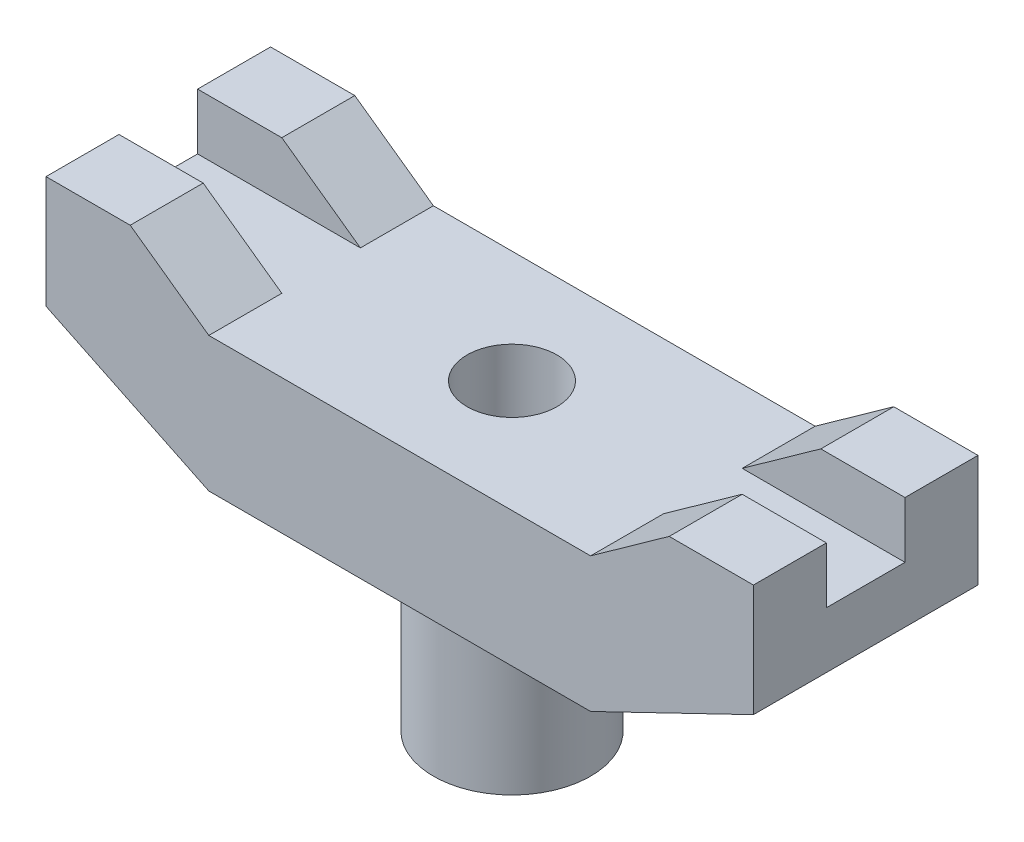
ISO-10303-21;
HEADER;
FILE_DESCRIPTION(('STEP AP214'),'2;1');
FILE_NAME('part.step','',(''),(''),'','','');
FILE_SCHEMA(('AUTOMOTIVE_DESIGN { 1 0 10303 214 1 1 1 1 }'));
ENDSEC;
DATA;
#1=APPLICATION_CONTEXT('core data for automotive mechanical design processes');
#2=APPLICATION_PROTOCOL_DEFINITION('international standard','automotive_design',2000,#1);
#3=PRODUCT_CONTEXT('',#1,'mechanical');
#4=PRODUCT('Part','Part','',(#3));
#5=PRODUCT_RELATED_PRODUCT_CATEGORY('part','',(#4));
#6=PRODUCT_DEFINITION_FORMATION('','',#4);
#7=PRODUCT_DEFINITION_CONTEXT('part definition',#1,'design');
#8=PRODUCT_DEFINITION('design','',#6,#7);
#9=PRODUCT_DEFINITION_SHAPE('','',#8);
#10=(LENGTH_UNIT() NAMED_UNIT(*) SI_UNIT(.MILLI.,.METRE.));
#11=(NAMED_UNIT(*) PLANE_ANGLE_UNIT() SI_UNIT($,.RADIAN.));
#12=(NAMED_UNIT(*) SI_UNIT($,.STERADIAN.) SOLID_ANGLE_UNIT());
#13=UNCERTAINTY_MEASURE_WITH_UNIT(LENGTH_MEASURE(1.E-05),#10,'distance_accuracy_value','');
#14=(GEOMETRIC_REPRESENTATION_CONTEXT(3) GLOBAL_UNCERTAINTY_ASSIGNED_CONTEXT((#13)) GLOBAL_UNIT_ASSIGNED_CONTEXT((#10,
#11,#12)) REPRESENTATION_CONTEXT('',''));
#15=CARTESIAN_POINT('',(0.,0.,0.));
#16=DIRECTION('',(0.,0.,1.));
#17=DIRECTION('',(1.,0.,0.));
#18=AXIS2_PLACEMENT_3D('',#15,#16,#17);
#19=CARTESIAN_POINT('',(0.,5.,0.));
#20=DIRECTION('',(0.,1.,0.));
#21=DIRECTION('',(0.,0.,1.));
#22=AXIS2_PLACEMENT_3D('',#19,#20,#21);
#23=PLANE('',#22);
#24=DIRECTION('',(-1.,0.,0.));
#25=VECTOR('',#24,1.);
#26=CARTESIAN_POINT('',(63.,5.,13.5));
#27=LINE('',#26,#25);
#28=CARTESIAN_POINT('',(7.5,5.,13.5));
#29=VERTEX_POINT('',#28);
#30=CARTESIAN_POINT('',(0.,5.,13.5));
#31=VERTEX_POINT('',#30);
#32=EDGE_CURVE('E211',#29,#31,#27,.T.);
#33=ORIENTED_EDGE('',*,*,#32,.T.);
#34=DIRECTION('',(0.,0.,1.));
#35=VECTOR('',#34,1.);
#36=CARTESIAN_POINT('',(0.,5.,0.));
#37=LINE('',#36,#35);
#38=CARTESIAN_POINT('',(0.,5.,20.));
#39=VERTEX_POINT('',#38);
#40=EDGE_CURVE('E257',#31,#39,#37,.T.);
#41=ORIENTED_EDGE('',*,*,#40,.T.);
#42=DIRECTION('',(-1.,0.,0.));
#43=VECTOR('',#42,1.);
#44=CARTESIAN_POINT('',(0.,5.,20.));
#45=LINE('',#44,#43);
#46=CARTESIAN_POINT('',(7.5,5.,20.));
#47=VERTEX_POINT('',#46);
#48=EDGE_CURVE('E248',#47,#39,#45,.T.);
#49=ORIENTED_EDGE('',*,*,#48,.F.);
#50=DIRECTION('',(0.,0.,1.));
#51=VECTOR('',#50,1.);
#52=CARTESIAN_POINT('',(7.5,5.,0.));
#53=LINE('',#52,#51);
#54=EDGE_CURVE('E262',#29,#47,#53,.T.);
#55=ORIENTED_EDGE('',*,*,#54,.F.);
#56=EDGE_LOOP('',(#33,#41,#49,#55));
#57=FACE_BOUND('',#56,.T.);
#58=ADVANCED_FACE('F44',(#57),#23,.T.);
#59=CARTESIAN_POINT('',(14.5,0.,0.));
#60=DIRECTION('',(0.581238193719096,0.813733471206735,0.));
#61=DIRECTION('',(-0.813733471206735,0.581238193719096,0.));
#62=AXIS2_PLACEMENT_3D('',#59,#60,#61);
#63=PLANE('',#62);
#64=DIRECTION('',(0.813733471206735,-0.581238193719096,0.));
#65=VECTOR('',#64,1.);
#66=CARTESIAN_POINT('',(14.5,0.,13.5));
#67=LINE('',#66,#65);
#68=CARTESIAN_POINT('',(14.5,0.,13.5));
#69=VERTEX_POINT('',#68);
#70=EDGE_CURVE('E219',#29,#69,#67,.T.);
#71=ORIENTED_EDGE('',*,*,#70,.F.);
#72=ORIENTED_EDGE('',*,*,#54,.T.);
#73=DIRECTION('',(-0.813733471206735,0.581238193719096,0.));
#74=VECTOR('',#73,1.);
#75=CARTESIAN_POINT('',(14.5,0.,20.));
#76=LINE('',#75,#74);
#77=CARTESIAN_POINT('',(14.5,0.,20.));
#78=VERTEX_POINT('',#77);
#79=EDGE_CURVE('E240',#78,#47,#76,.T.);
#80=ORIENTED_EDGE('',*,*,#79,.F.);
#81=DIRECTION('',(0.,0.,1.));
#82=VECTOR('',#81,1.);
#83=CARTESIAN_POINT('',(14.5,0.,0.));
#84=LINE('',#83,#82);
#85=EDGE_CURVE('E253',#69,#78,#84,.T.);
#86=ORIENTED_EDGE('',*,*,#85,.F.);
#87=EDGE_LOOP('',(#71,#72,#80,#86));
#88=FACE_BOUND('',#87,.T.);
#89=ADVANCED_FACE('F343',(#88),#63,.T.);
#90=CARTESIAN_POINT('',(48.5,0.,0.));
#91=DIRECTION('',(-0.581238193719096,0.813733471206735,0.));
#92=DIRECTION('',(-0.813733471206735,-0.581238193719096,0.));
#93=AXIS2_PLACEMENT_3D('',#90,#91,#92);
#94=PLANE('',#93);
#95=DIRECTION('',(0.813733471206735,0.581238193719096,0.));
#96=VECTOR('',#95,1.);
#97=CARTESIAN_POINT('',(48.5,0.,13.5));
#98=LINE('',#97,#96);
#99=CARTESIAN_POINT('',(48.5,0.,13.5));
#100=VERTEX_POINT('',#99);
#101=CARTESIAN_POINT('',(55.5,5.,13.5));
#102=VERTEX_POINT('',#101);
#103=EDGE_CURVE('E217',#100,#102,#98,.T.);
#104=ORIENTED_EDGE('',*,*,#103,.F.);
#105=DIRECTION('',(0.,0.,1.));
#106=VECTOR('',#105,1.);
#107=CARTESIAN_POINT('',(48.5,0.,0.));
#108=LINE('',#107,#106);
#109=CARTESIAN_POINT('',(48.5,0.,20.));
#110=VERTEX_POINT('',#109);
#111=EDGE_CURVE('E236',#100,#110,#108,.T.);
#112=ORIENTED_EDGE('',*,*,#111,.T.);
#113=DIRECTION('',(-0.813733471206735,-0.581238193719096,0.));
#114=VECTOR('',#113,1.);
#115=CARTESIAN_POINT('',(48.5,0.,20.));
#116=LINE('',#115,#114);
#117=CARTESIAN_POINT('',(55.5,5.,20.));
#118=VERTEX_POINT('',#117);
#119=EDGE_CURVE('E230',#118,#110,#116,.T.);
#120=ORIENTED_EDGE('',*,*,#119,.F.);
#121=DIRECTION('',(0.,0.,1.));
#122=VECTOR('',#121,1.);
#123=CARTESIAN_POINT('',(55.5,5.,0.));
#124=LINE('',#123,#122);
#125=EDGE_CURVE('E245',#102,#118,#124,.T.);
#126=ORIENTED_EDGE('',*,*,#125,.F.);
#127=EDGE_LOOP('',(#104,#112,#120,#126));
#128=FACE_BOUND('',#127,.T.);
#129=ADVANCED_FACE('F348',(#128),#94,.T.);
#130=CARTESIAN_POINT('',(63.,5.,0.));
#131=DIRECTION('',(0.,1.,0.));
#132=DIRECTION('',(0.,0.,1.));
#133=AXIS2_PLACEMENT_3D('',#130,#131,#132);
#134=PLANE('',#133);
#135=CARTESIAN_POINT('',(63.,5.,13.5));
#136=VERTEX_POINT('',#135);
#137=EDGE_CURVE('E208',#136,#102,#27,.T.);
#138=ORIENTED_EDGE('',*,*,#137,.T.);
#139=ORIENTED_EDGE('',*,*,#125,.T.);
#140=DIRECTION('',(-1.,0.,0.));
#141=VECTOR('',#140,1.);
#142=CARTESIAN_POINT('',(63.,5.,20.));
#143=LINE('',#142,#141);
#144=CARTESIAN_POINT('',(63.,5.,20.));
#145=VERTEX_POINT('',#144);
#146=EDGE_CURVE('E225',#145,#118,#143,.T.);
#147=ORIENTED_EDGE('',*,*,#146,.F.);
#148=DIRECTION('',(0.,0.,1.));
#149=VECTOR('',#148,1.);
#150=CARTESIAN_POINT('',(63.,5.,0.));
#151=LINE('',#150,#149);
#152=EDGE_CURVE('E229',#136,#145,#151,.T.);
#153=ORIENTED_EDGE('',*,*,#152,.F.);
#154=EDGE_LOOP('',(#138,#139,#147,#153));
#155=FACE_BOUND('',#154,.T.);
#156=ADVANCED_FACE('F354',(#155),#134,.T.);
#157=CARTESIAN_POINT('',(0.,0.,20.));
#158=DIRECTION('',(1.,0.,0.));
#159=DIRECTION('',(0.,0.,-1.));
#160=AXIS2_PLACEMENT_3D('',#157,#158,#159);
#161=PLANE('',#160);
#162=ORIENTED_EDGE('',*,*,#40,.F.);
#163=DIRECTION('',(0.,1.,0.));
#164=VECTOR('',#163,1.);
#165=CARTESIAN_POINT('',(0.,0.,13.5));
#166=LINE('',#165,#164);
#167=CARTESIAN_POINT('',(0.,0.,13.5));
#168=VERTEX_POINT('',#167);
#169=EDGE_CURVE('E191',#168,#31,#166,.T.);
#170=ORIENTED_EDGE('',*,*,#169,.F.);
#171=DIRECTION('',(0.,0.,1.));
#172=VECTOR('',#171,1.);
#173=CARTESIAN_POINT('',(0.,0.,6.5));
#174=LINE('',#173,#172);
#175=CARTESIAN_POINT('',(0.,0.,6.5));
#176=VERTEX_POINT('',#175);
#177=EDGE_CURVE('E197',#176,#168,#174,.T.);
#178=ORIENTED_EDGE('',*,*,#177,.F.);
#179=DIRECTION('',(0.,-1.,0.));
#180=VECTOR('',#179,1.);
#181=CARTESIAN_POINT('',(0.,5.,6.5));
#182=LINE('',#181,#180);
#183=CARTESIAN_POINT('',(0.,5.,6.5));
#184=VERTEX_POINT('',#183);
#185=EDGE_CURVE('E201',#184,#176,#182,.T.);
#186=ORIENTED_EDGE('',*,*,#185,.F.);
#187=CARTESIAN_POINT('',(0.,5.,0.));
#188=VERTEX_POINT('',#187);
#189=EDGE_CURVE('E258',#188,#184,#37,.T.);
#190=ORIENTED_EDGE('',*,*,#189,.F.);
#191=DIRECTION('',(0.,-1.,0.));
#192=VECTOR('',#191,1.);
#193=CARTESIAN_POINT('',(0.,0.,0.));
#194=LINE('',#193,#192);
#195=CARTESIAN_POINT('',(0.,-5.,0.));
#196=VERTEX_POINT('',#195);
#197=EDGE_CURVE('E259',#188,#196,#194,.T.);
#198=ORIENTED_EDGE('',*,*,#197,.T.);
#199=DIRECTION('',(0.,0.,-1.));
#200=VECTOR('',#199,1.);
#201=CARTESIAN_POINT('',(0.,-5.,20.));
#202=LINE('',#201,#200);
#203=CARTESIAN_POINT('',(0.,-5.,20.));
#204=VERTEX_POINT('',#203);
#205=EDGE_CURVE('E53',#204,#196,#202,.T.);
#206=ORIENTED_EDGE('',*,*,#205,.F.);
#207=DIRECTION('',(0.,-1.,0.));
#208=VECTOR('',#207,1.);
#209=CARTESIAN_POINT('',(0.,0.,20.));
#210=LINE('',#209,#208);
#211=EDGE_CURVE('E270',#39,#204,#210,.T.);
#212=ORIENTED_EDGE('',*,*,#211,.F.);
#213=EDGE_LOOP('',(#162,#170,#178,#186,#190,#198,#206,#212));
#214=FACE_BOUND('',#213,.T.);
#215=ADVANCED_FACE('F50',(#214),#161,.F.);
#216=CARTESIAN_POINT('',(0.,-5.,20.));
#217=DIRECTION('',(0.434749065831176,0.900551636364578,0.));
#218=DIRECTION('',(-0.900551636364579,0.434749065831176,0.));
#219=AXIS2_PLACEMENT_3D('',#216,#217,#218);
#220=PLANE('',#219);
#221=DIRECTION('',(0.900551636364578,-0.434749065831176,0.));
#222=VECTOR('',#221,1.);
#223=CARTESIAN_POINT('',(0.,-5.,0.));
#224=LINE('',#223,#222);
#225=CARTESIAN_POINT('',(14.5,-12.,0.));
#226=VERTEX_POINT('',#225);
#227=EDGE_CURVE('E287',#196,#226,#224,.T.);
#228=ORIENTED_EDGE('',*,*,#227,.T.);
#229=DIRECTION('',(0.,0.,-1.));
#230=VECTOR('',#229,1.);
#231=CARTESIAN_POINT('',(14.5,-12.,20.));
#232=LINE('',#231,#230);
#233=CARTESIAN_POINT('',(14.5,-12.,20.));
#234=VERTEX_POINT('',#233);
#235=EDGE_CURVE('E302',#234,#226,#232,.T.);
#236=ORIENTED_EDGE('',*,*,#235,.F.);
#237=DIRECTION('',(0.900551636364578,-0.434749065831176,0.));
#238=VECTOR('',#237,1.);
#239=CARTESIAN_POINT('',(0.,-5.,20.));
#240=LINE('',#239,#238);
#241=EDGE_CURVE('E269',#204,#234,#240,.T.);
#242=ORIENTED_EDGE('',*,*,#241,.F.);
#243=ORIENTED_EDGE('',*,*,#205,.T.);
#244=EDGE_LOOP('',(#228,#236,#242,#243));
#245=FACE_BOUND('',#244,.T.);
#246=ADVANCED_FACE('F308',(#245),#220,.F.);
#247=CARTESIAN_POINT('',(31.5,-12.,20.));
#248=DIRECTION('',(0.,1.,0.));
#249=DIRECTION('',(0.,0.,1.));
#250=AXIS2_PLACEMENT_3D('',#247,#248,#249);
#251=PLANE('',#250);
#252=CARTESIAN_POINT('',(31.5,-12.,10.));
#253=DIRECTION('',(0.,-1.,0.));
#254=DIRECTION('',(0.,0.,-1.));
#255=AXIS2_PLACEMENT_3D('',#252,#253,#254);
#256=CIRCLE('',#255,7.);
#257=CARTESIAN_POINT('',(31.5,-12.,3.));
#258=VERTEX_POINT('',#257);
#259=EDGE_CURVE('E11',#258,#258,#256,.T.);
#260=ORIENTED_EDGE('',*,*,#259,.F.);
#261=EDGE_LOOP('',(#260));
#262=FACE_BOUND('',#261,.T.);
#263=DIRECTION('',(1.,0.,0.));
#264=VECTOR('',#263,1.);
#265=CARTESIAN_POINT('',(31.5,-12.,0.));
#266=LINE('',#265,#264);
#267=CARTESIAN_POINT('',(48.5,-12.,0.));
#268=VERTEX_POINT('',#267);
#269=EDGE_CURVE('E289',#226,#268,#266,.T.);
#270=ORIENTED_EDGE('',*,*,#269,.T.);
#271=DIRECTION('',(0.,0.,-1.));
#272=VECTOR('',#271,1.);
#273=CARTESIAN_POINT('',(48.5,-12.,20.));
#274=LINE('',#273,#272);
#275=CARTESIAN_POINT('',(48.5,-12.,20.));
#276=VERTEX_POINT('',#275);
#277=EDGE_CURVE('E296',#276,#268,#274,.T.);
#278=ORIENTED_EDGE('',*,*,#277,.F.);
#279=DIRECTION('',(1.,0.,0.));
#280=VECTOR('',#279,1.);
#281=CARTESIAN_POINT('',(31.5,-12.,20.));
#282=LINE('',#281,#280);
#283=EDGE_CURVE('E272',#234,#276,#282,.T.);
#284=ORIENTED_EDGE('',*,*,#283,.F.);
#285=ORIENTED_EDGE('',*,*,#235,.T.);
#286=EDGE_LOOP('',(#270,#278,#284,#285));
#287=FACE_BOUND('',#286,.T.);
#288=ADVANCED_FACE('F321',(#262,#287),#251,.F.);
#289=CARTESIAN_POINT('',(63.,-5.,20.));
#290=DIRECTION('',(-0.434749065831176,0.900551636364578,0.));
#291=DIRECTION('',(-0.900551636364579,-0.434749065831176,0.));
#292=AXIS2_PLACEMENT_3D('',#289,#290,#291);
#293=PLANE('',#292);
#294=DIRECTION('',(0.900551636364578,0.434749065831176,0.));
#295=VECTOR('',#294,1.);
#296=CARTESIAN_POINT('',(63.,-5.,0.));
#297=LINE('',#296,#295);
#298=CARTESIAN_POINT('',(63.,-5.,0.));
#299=VERTEX_POINT('',#298);
#300=EDGE_CURVE('E292',#268,#299,#297,.T.);
#301=ORIENTED_EDGE('',*,*,#300,.T.);
#302=DIRECTION('',(0.,0.,-1.));
#303=VECTOR('',#302,1.);
#304=CARTESIAN_POINT('',(63.,-5.,20.));
#305=LINE('',#304,#303);
#306=CARTESIAN_POINT('',(63.,-5.,20.));
#307=VERTEX_POINT('',#306);
#308=EDGE_CURVE('E281',#307,#299,#305,.T.);
#309=ORIENTED_EDGE('',*,*,#308,.F.);
#310=DIRECTION('',(0.900551636364578,0.434749065831176,0.));
#311=VECTOR('',#310,1.);
#312=CARTESIAN_POINT('',(63.,-5.,20.));
#313=LINE('',#312,#311);
#314=EDGE_CURVE('E274',#276,#307,#313,.T.);
#315=ORIENTED_EDGE('',*,*,#314,.F.);
#316=ORIENTED_EDGE('',*,*,#277,.T.);
#317=EDGE_LOOP('',(#301,#309,#315,#316));
#318=FACE_BOUND('',#317,.T.);
#319=ADVANCED_FACE('F324',(#318),#293,.F.);
#320=CARTESIAN_POINT('',(63.,0.,20.));
#321=DIRECTION('',(-1.,0.,0.));
#322=DIRECTION('',(0.,0.,1.));
#323=AXIS2_PLACEMENT_3D('',#320,#321,#322);
#324=PLANE('',#323);
#325=DIRECTION('',(0.,0.,1.));
#326=VECTOR('',#325,1.);
#327=CARTESIAN_POINT('',(63.,0.,6.5));
#328=LINE('',#327,#326);
#329=CARTESIAN_POINT('',(63.,0.,6.5));
#330=VERTEX_POINT('',#329);
#331=CARTESIAN_POINT('',(63.,0.,13.5));
#332=VERTEX_POINT('',#331);
#333=EDGE_CURVE('E182',#330,#332,#328,.T.);
#334=ORIENTED_EDGE('',*,*,#333,.T.);
#335=DIRECTION('',(0.,1.,0.));
#336=VECTOR('',#335,1.);
#337=CARTESIAN_POINT('',(63.,0.,13.5));
#338=LINE('',#337,#336);
#339=EDGE_CURVE('E187',#332,#136,#338,.T.);
#340=ORIENTED_EDGE('',*,*,#339,.T.);
#341=ORIENTED_EDGE('',*,*,#152,.T.);
#342=DIRECTION('',(0.,1.,0.));
#343=VECTOR('',#342,1.);
#344=CARTESIAN_POINT('',(63.,0.,20.));
#345=LINE('',#344,#343);
#346=EDGE_CURVE('E280',#307,#145,#345,.T.);
#347=ORIENTED_EDGE('',*,*,#346,.F.);
#348=ORIENTED_EDGE('',*,*,#308,.T.);
#349=DIRECTION('',(0.,1.,0.));
#350=VECTOR('',#349,1.);
#351=CARTESIAN_POINT('',(63.,0.,0.));
#352=LINE('',#351,#350);
#353=CARTESIAN_POINT('',(63.,5.,0.));
#354=VERTEX_POINT('',#353);
#355=EDGE_CURVE('E291',#299,#354,#352,.T.);
#356=ORIENTED_EDGE('',*,*,#355,.T.);
#357=CARTESIAN_POINT('',(63.,5.,6.5));
#358=VERTEX_POINT('',#357);
#359=EDGE_CURVE('E194',#354,#358,#151,.T.);
#360=ORIENTED_EDGE('',*,*,#359,.T.);
#361=DIRECTION('',(0.,-1.,0.));
#362=VECTOR('',#361,1.);
#363=CARTESIAN_POINT('',(63.,5.,6.5));
#364=LINE('',#363,#362);
#365=EDGE_CURVE('E66',#358,#330,#364,.T.);
#366=ORIENTED_EDGE('',*,*,#365,.T.);
#367=EDGE_LOOP('',(#334,#340,#341,#347,#348,#356,#360,#366));
#368=FACE_BOUND('',#367,.T.);
#369=ADVANCED_FACE('F195',(#368),#324,.F.);
#370=CARTESIAN_POINT('',(0.,0.,20.));
#371=DIRECTION('',(0.,-1.,0.));
#372=DIRECTION('',(0.,0.,-1.));
#373=AXIS2_PLACEMENT_3D('',#370,#371,#372);
#374=PLANE('',#373);
#375=CARTESIAN_POINT('',(31.5,0.,10.));
#376=DIRECTION('',(0.,1.,0.));
#377=DIRECTION('',(0.,0.,1.));
#378=AXIS2_PLACEMENT_3D('',#375,#376,#377);
#379=CIRCLE('',#378,4.);
#380=CARTESIAN_POINT('',(31.5,0.,14.));
#381=VERTEX_POINT('',#380);
#382=EDGE_CURVE('E440',#381,#381,#379,.T.);
#383=ORIENTED_EDGE('',*,*,#382,.F.);
#384=EDGE_LOOP('',(#383));
#385=FACE_BOUND('',#384,.T.);
#386=CARTESIAN_POINT('',(14.5,0.,0.));
#387=VERTEX_POINT('',#386);
#388=CARTESIAN_POINT('',(14.5,0.,6.5));
#389=VERTEX_POINT('',#388);
#390=EDGE_CURVE('E264',#387,#389,#84,.T.);
#391=ORIENTED_EDGE('',*,*,#390,.T.);
#392=DIRECTION('',(-1.,0.,0.));
#393=VECTOR('',#392,1.);
#394=CARTESIAN_POINT('',(63.,0.,6.5));
#395=LINE('',#394,#393);
#396=EDGE_CURVE('E65',#389,#176,#395,.T.);
#397=ORIENTED_EDGE('',*,*,#396,.T.);
#398=ORIENTED_EDGE('',*,*,#177,.T.);
#399=DIRECTION('',(-1.,0.,0.));
#400=VECTOR('',#399,1.);
#401=CARTESIAN_POINT('',(63.,0.,13.5));
#402=LINE('',#401,#400);
#403=EDGE_CURVE('E178',#69,#168,#402,.T.);
#404=ORIENTED_EDGE('',*,*,#403,.F.);
#405=ORIENTED_EDGE('',*,*,#85,.T.);
#406=DIRECTION('',(-1.,0.,0.));
#407=VECTOR('',#406,1.);
#408=CARTESIAN_POINT('',(0.,0.,20.));
#409=LINE('',#408,#407);
#410=EDGE_CURVE('E278',#110,#78,#409,.T.);
#411=ORIENTED_EDGE('',*,*,#410,.F.);
#412=ORIENTED_EDGE('',*,*,#111,.F.);
#413=EDGE_CURVE('E183',#332,#100,#402,.T.);
#414=ORIENTED_EDGE('',*,*,#413,.F.);
#415=ORIENTED_EDGE('',*,*,#333,.F.);
#416=CARTESIAN_POINT('',(48.5,0.,6.5));
#417=VERTEX_POINT('',#416);
#418=EDGE_CURVE('E168',#330,#417,#395,.T.);
#419=ORIENTED_EDGE('',*,*,#418,.T.);
#420=CARTESIAN_POINT('',(48.5,0.,0.));
#421=VERTEX_POINT('',#420);
#422=EDGE_CURVE('E231',#421,#417,#108,.T.);
#423=ORIENTED_EDGE('',*,*,#422,.F.);
#424=DIRECTION('',(-1.,0.,0.));
#425=VECTOR('',#424,1.);
#426=CARTESIAN_POINT('',(0.,0.,0.));
#427=LINE('',#426,#425);
#428=EDGE_CURVE('E271',#421,#387,#427,.T.);
#429=ORIENTED_EDGE('',*,*,#428,.T.);
#430=EDGE_LOOP('',(#391,#397,#398,#404,#405,#411,#412,#414,#415,#419,#423,#429));
#431=FACE_BOUND('',#430,.T.);
#432=ADVANCED_FACE('F181',(#385,#431),#374,.F.);
#433=CARTESIAN_POINT('',(0.,0.,20.));
#434=DIRECTION('',(0.,0.,-1.));
#435=DIRECTION('',(-1.,0.,0.));
#436=AXIS2_PLACEMENT_3D('',#433,#434,#435);
#437=PLANE('',#436);
#438=ORIENTED_EDGE('',*,*,#211,.T.);
#439=ORIENTED_EDGE('',*,*,#241,.T.);
#440=ORIENTED_EDGE('',*,*,#283,.T.);
#441=ORIENTED_EDGE('',*,*,#314,.T.);
#442=ORIENTED_EDGE('',*,*,#346,.T.);
#443=ORIENTED_EDGE('',*,*,#146,.T.);
#444=ORIENTED_EDGE('',*,*,#119,.T.);
#445=ORIENTED_EDGE('',*,*,#410,.T.);
#446=ORIENTED_EDGE('',*,*,#79,.T.);
#447=ORIENTED_EDGE('',*,*,#48,.T.);
#448=EDGE_LOOP('',(#438,#439,#440,#441,#442,#443,#444,#445,#446,#447));
#449=FACE_BOUND('',#448,.T.);
#450=ADVANCED_FACE('F328',(#449),#437,.F.);
#451=CARTESIAN_POINT('',(0.,0.,0.));
#452=DIRECTION('',(0.,0.,-1.));
#453=DIRECTION('',(-1.,0.,0.));
#454=AXIS2_PLACEMENT_3D('',#451,#452,#453);
#455=PLANE('',#454);
#456=ORIENTED_EDGE('',*,*,#197,.F.);
#457=DIRECTION('',(-1.,0.,0.));
#458=VECTOR('',#457,1.);
#459=CARTESIAN_POINT('',(0.,5.,0.));
#460=LINE('',#459,#458);
#461=CARTESIAN_POINT('',(7.5,5.,0.));
#462=VERTEX_POINT('',#461);
#463=EDGE_CURVE('E250',#462,#188,#460,.T.);
#464=ORIENTED_EDGE('',*,*,#463,.F.);
#465=DIRECTION('',(-0.813733471206735,0.581238193719096,0.));
#466=VECTOR('',#465,1.);
#467=CARTESIAN_POINT('',(14.5,0.,0.));
#468=LINE('',#467,#466);
#469=EDGE_CURVE('E242',#387,#462,#468,.T.);
#470=ORIENTED_EDGE('',*,*,#469,.F.);
#471=ORIENTED_EDGE('',*,*,#428,.F.);
#472=DIRECTION('',(-0.813733471206735,-0.581238193719096,0.));
#473=VECTOR('',#472,1.);
#474=CARTESIAN_POINT('',(48.5,0.,0.));
#475=LINE('',#474,#473);
#476=CARTESIAN_POINT('',(55.5,5.,0.));
#477=VERTEX_POINT('',#476);
#478=EDGE_CURVE('E228',#477,#421,#475,.T.);
#479=ORIENTED_EDGE('',*,*,#478,.F.);
#480=DIRECTION('',(-1.,0.,0.));
#481=VECTOR('',#480,1.);
#482=CARTESIAN_POINT('',(63.,5.,0.));
#483=LINE('',#482,#481);
#484=EDGE_CURVE('E224',#354,#477,#483,.T.);
#485=ORIENTED_EDGE('',*,*,#484,.F.);
#486=ORIENTED_EDGE('',*,*,#355,.F.);
#487=ORIENTED_EDGE('',*,*,#300,.F.);
#488=ORIENTED_EDGE('',*,*,#269,.F.);
#489=ORIENTED_EDGE('',*,*,#227,.F.);
#490=EDGE_LOOP('',(#456,#464,#470,#471,#479,#485,#486,#487,#488,#489));
#491=FACE_BOUND('',#490,.T.);
#492=ADVANCED_FACE('F312',(#491),#455,.T.);
#493=DIRECTION('',(-1.,0.,0.));
#494=VECTOR('',#493,1.);
#495=CARTESIAN_POINT('',(63.,5.,6.5));
#496=LINE('',#495,#494);
#497=CARTESIAN_POINT('',(7.5,5.,6.5));
#498=VERTEX_POINT('',#497);
#499=EDGE_CURVE('E205',#498,#184,#496,.T.);
#500=ORIENTED_EDGE('',*,*,#499,.F.);
#501=EDGE_CURVE('E261',#462,#498,#53,.T.);
#502=ORIENTED_EDGE('',*,*,#501,.F.);
#503=ORIENTED_EDGE('',*,*,#463,.T.);
#504=ORIENTED_EDGE('',*,*,#189,.T.);
#505=EDGE_LOOP('',(#500,#502,#503,#504));
#506=FACE_BOUND('',#505,.T.);
#507=ADVANCED_FACE('F366',(#506),#23,.T.);
#508=DIRECTION('',(-0.813733471206735,0.581238193719096,0.));
#509=VECTOR('',#508,1.);
#510=CARTESIAN_POINT('',(14.5,0.,6.5));
#511=LINE('',#510,#509);
#512=EDGE_CURVE('E216',#389,#498,#511,.T.);
#513=ORIENTED_EDGE('',*,*,#512,.F.);
#514=ORIENTED_EDGE('',*,*,#390,.F.);
#515=ORIENTED_EDGE('',*,*,#469,.T.);
#516=ORIENTED_EDGE('',*,*,#501,.T.);
#517=EDGE_LOOP('',(#513,#514,#515,#516));
#518=FACE_BOUND('',#517,.T.);
#519=ADVANCED_FACE('F365',(#518),#63,.T.);
#520=DIRECTION('',(-0.813733471206735,-0.581238193719096,0.));
#521=VECTOR('',#520,1.);
#522=CARTESIAN_POINT('',(48.5,0.,6.5));
#523=LINE('',#522,#521);
#524=CARTESIAN_POINT('',(55.5,5.,6.5));
#525=VERTEX_POINT('',#524);
#526=EDGE_CURVE('E172',#525,#417,#523,.T.);
#527=ORIENTED_EDGE('',*,*,#526,.F.);
#528=EDGE_CURVE('E239',#477,#525,#124,.T.);
#529=ORIENTED_EDGE('',*,*,#528,.F.);
#530=ORIENTED_EDGE('',*,*,#478,.T.);
#531=ORIENTED_EDGE('',*,*,#422,.T.);
#532=EDGE_LOOP('',(#527,#529,#530,#531));
#533=FACE_BOUND('',#532,.T.);
#534=ADVANCED_FACE('F363',(#533),#94,.T.);
#535=EDGE_CURVE('E213',#358,#525,#496,.T.);
#536=ORIENTED_EDGE('',*,*,#535,.F.);
#537=ORIENTED_EDGE('',*,*,#359,.F.);
#538=ORIENTED_EDGE('',*,*,#484,.T.);
#539=ORIENTED_EDGE('',*,*,#528,.T.);
#540=EDGE_LOOP('',(#536,#537,#538,#539));
#541=FACE_BOUND('',#540,.T.);
#542=ADVANCED_FACE('F359',(#541),#134,.T.);
#543=CARTESIAN_POINT('',(63.,0.,13.5));
#544=DIRECTION('',(0.,0.,1.));
#545=DIRECTION('',(1.,0.,0.));
#546=AXIS2_PLACEMENT_3D('',#543,#544,#545);
#547=PLANE('',#546);
#548=ORIENTED_EDGE('',*,*,#103,.T.);
#549=ORIENTED_EDGE('',*,*,#137,.F.);
#550=ORIENTED_EDGE('',*,*,#339,.F.);
#551=ORIENTED_EDGE('',*,*,#413,.T.);
#552=EDGE_LOOP('',(#548,#549,#550,#551));
#553=FACE_BOUND('',#552,.T.);
#554=ADVANCED_FACE('F355',(#553),#547,.F.);
#555=CARTESIAN_POINT('',(63.,5.,6.5));
#556=DIRECTION('',(0.,0.,-1.));
#557=DIRECTION('',(-1.,0.,0.));
#558=AXIS2_PLACEMENT_3D('',#555,#556,#557);
#559=PLANE('',#558);
#560=ORIENTED_EDGE('',*,*,#526,.T.);
#561=ORIENTED_EDGE('',*,*,#418,.F.);
#562=ORIENTED_EDGE('',*,*,#365,.F.);
#563=ORIENTED_EDGE('',*,*,#535,.T.);
#564=EDGE_LOOP('',(#560,#561,#562,#563));
#565=FACE_BOUND('',#564,.T.);
#566=ADVANCED_FACE('F175',(#565),#559,.F.);
#567=ORIENTED_EDGE('',*,*,#70,.T.);
#568=ORIENTED_EDGE('',*,*,#403,.T.);
#569=ORIENTED_EDGE('',*,*,#169,.T.);
#570=ORIENTED_EDGE('',*,*,#32,.F.);
#571=EDGE_LOOP('',(#567,#568,#569,#570));
#572=FACE_BOUND('',#571,.T.);
#573=ADVANCED_FACE('F337',(#572),#547,.F.);
#574=ORIENTED_EDGE('',*,*,#512,.T.);
#575=ORIENTED_EDGE('',*,*,#499,.T.);
#576=ORIENTED_EDGE('',*,*,#185,.T.);
#577=ORIENTED_EDGE('',*,*,#396,.F.);
#578=EDGE_LOOP('',(#574,#575,#576,#577));
#579=FACE_BOUND('',#578,.T.);
#580=ADVANCED_FACE('F368',(#579),#559,.F.);
#581=CARTESIAN_POINT('',(31.5,-27.,10.));
#582=DIRECTION('',(0.,1.,0.));
#583=DIRECTION('',(0.,0.,1.));
#584=AXIS2_PLACEMENT_3D('',#581,#582,#583);
#585=CYLINDRICAL_SURFACE('',#584,7.);
#586=CARTESIAN_POINT('',(31.5,-27.,10.));
#587=DIRECTION('',(0.,-1.,0.));
#588=DIRECTION('',(0.,0.,-1.));
#589=AXIS2_PLACEMENT_3D('',#586,#587,#588);
#590=CIRCLE('',#589,7.);
#591=CARTESIAN_POINT('',(31.5,-27.,3.));
#592=VERTEX_POINT('',#591);
#593=EDGE_CURVE('E202',#592,#592,#590,.T.);
#594=ORIENTED_EDGE('',*,*,#593,.F.);
#595=EDGE_LOOP('',(#594));
#596=FACE_BOUND('',#595,.T.);
#597=ORIENTED_EDGE('',*,*,#259,.T.);
#598=EDGE_LOOP('',(#597));
#599=FACE_BOUND('',#598,.T.);
#600=ADVANCED_FACE('F420',(#596,#599),#585,.T.);
#601=CARTESIAN_POINT('',(31.5,-27.,10.));
#602=DIRECTION('',(0.,-1.,0.));
#603=DIRECTION('',(0.,0.,-1.));
#604=AXIS2_PLACEMENT_3D('',#601,#602,#603);
#605=PLANE('',#604);
#606=CARTESIAN_POINT('',(31.5,-27.,10.));
#607=DIRECTION('',(0.,-1.,0.));
#608=DIRECTION('',(0.,0.,-1.));
#609=AXIS2_PLACEMENT_3D('',#606,#607,#608);
#610=CIRCLE('',#609,4.);
#611=CARTESIAN_POINT('',(31.5,-27.,6.));
#612=VERTEX_POINT('',#611);
#613=EDGE_CURVE('E47',#612,#612,#610,.T.);
#614=ORIENTED_EDGE('',*,*,#613,.F.);
#615=EDGE_LOOP('',(#614));
#616=FACE_BOUND('',#615,.T.);
#617=ORIENTED_EDGE('',*,*,#593,.T.);
#618=EDGE_LOOP('',(#617));
#619=FACE_BOUND('',#618,.T.);
#620=ADVANCED_FACE('F425',(#616,#619),#605,.T.);
#621=CARTESIAN_POINT('',(31.5,-32.,10.));
#622=DIRECTION('',(0.,1.,0.));
#623=DIRECTION('',(0.,0.,1.));
#624=AXIS2_PLACEMENT_3D('',#621,#622,#623);
#625=CYLINDRICAL_SURFACE('',#624,4.);
#626=ORIENTED_EDGE('',*,*,#613,.T.);
#627=EDGE_LOOP('',(#626));
#628=FACE_BOUND('',#627,.T.);
#629=ORIENTED_EDGE('',*,*,#382,.T.);
#630=EDGE_LOOP('',(#629));
#631=FACE_BOUND('',#630,.T.);
#632=ADVANCED_FACE('F426',(#628,#631),#625,.F.);
#633=CLOSED_SHELL('',(#58,#89,#129,#156,#215,#246,#288,#319,#369,#432,#450,#492,#507,#519,#534,
#542,#554,#566,#573,#580,#600,#620,#632));
#634=MANIFOLD_SOLID_BREP('B2',#633);
#635=ADVANCED_BREP_SHAPE_REPRESENTATION('',(#18,#634),#14);
#636=SHAPE_DEFINITION_REPRESENTATION(#9,#635);
ENDSEC;
END-ISO-10303-21;
